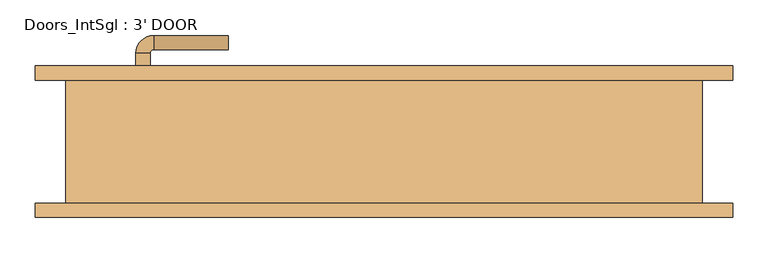
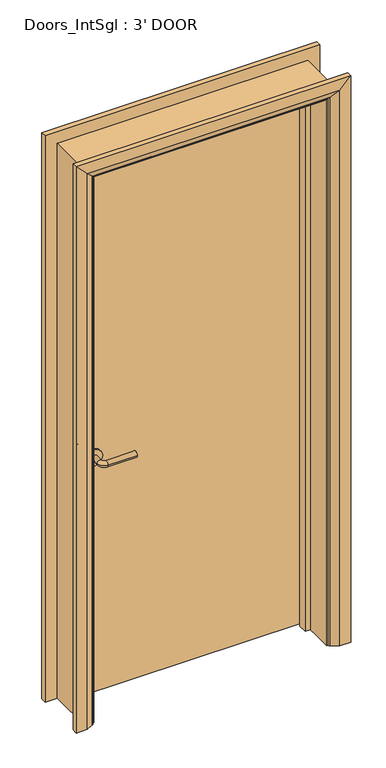
"""IFC4 building model written with IfcOpenShell, lengths in millimetres: door geometry, Doors_IntSgl : 3' DOOR."""

from ifc_helpers import new_model, si_unit, point, frame, frame_2d, origin, place, context, project, spatial, polyline, circle_curve, ellipse_curve, trimmed, segment, composite_curve, outline, extrude, faceted_brep, source, transform, mapped, element, save
from ifc_brep_helpers import plane_surface, cylinder_surface, revolved_surface, advanced_brep


def doors_intsgl_3_door_f61d7fb9(model_context):
    return source(origin(), model_context, "Body", "SolidModel", [
        advanced_brep(
        [(-350.2, 40.868, 900.0), (-330.2, 40.868, 900.0), (-330.2, 10.868, 900.0), (-350.2, 10.868, 900.0), (-325.2, 5.868, 900.0), (-325.2, -14.132, 900.0), (-220.2, -14.132, 900.0), (-220.2, 5.868, 900.0)],
        [
            (0, 1, circle_curve(frame((-340.2, 40.868, 900.0), z_axis=(0.0, 1.0, 0.0), x_axis=(1.0, 0.0, 0.0)), 10.0)),
            (1, 0, circle_curve(frame((-340.2, 40.868, 900.0), z_axis=(0.0, 1.0, 0.0), x_axis=(1.0, 0.0, 0.0)), 10.0)),
            (1, 2),
            (2, 3, circle_curve(frame((-340.2, 10.868, 900.0), z_axis=(0.0, 1.0, 0.0), x_axis=(1.0, 0.0, 0.0)), 10.0)),
            (3, 0),
            (3, 2, circle_curve(frame((-340.2, 10.868, 900.0), z_axis=(0.0, 1.0, 0.0), x_axis=(1.0, 0.0, 0.0)), 10.0)),
            (4, 5, circle_curve(frame((-325.2, -4.132, 900.0), z_axis=(-1.0, 0.0, 0.0), x_axis=(0.0, 1.0, 0.0)), 10.0)),
            (5, 3, circle_curve(frame((-325.2, 10.868, 900.0), z_axis=(0.0, 0.0, -1.0), x_axis=(-1.0, 0.0, 0.0)), 25.0)),
            (2, 4, circle_curve(frame((-325.2, 10.868, 900.0), z_axis=(0.0, 0.0, 1.0), x_axis=(-1.0, 0.0, 0.0)), 5.0)),
            (5, 4, circle_curve(frame((-325.2, -4.132, 900.0), z_axis=(-1.0, 0.0, 0.0), x_axis=(0.0, 1.0, 0.0)), 10.0)),
            (6, 7, circle_curve(frame((-220.2, -4.132, 900.0), z_axis=(1.0, 0.0, 0.0), x_axis=(0.0, 1.0, 0.0)), 10.0)),
            (7, 6, circle_curve(frame((-220.2, -4.132, 900.0), z_axis=(1.0, 0.0, 0.0), x_axis=(0.0, 1.0, 0.0)), 10.0)),
            (4, 7),
            (6, 5),
        ],
        [
            plane_surface(frame((-340.2, 40.868, 900.0), z_axis=(0.0, 1.0, 0.0), x_axis=(0.0, 0.0, 1.0))),
            cylinder_surface(frame((-340.2, 40.868, 900.0), z_axis=(0.0, 1.0, 0.0), x_axis=(1.0, 0.0, 0.0)), 10.0),
            revolved_surface(trimmed(ellipse_curve(frame((-340.2, 10.868, 900.0), z_axis=(0.0, -1.0, 0.0), x_axis=(1.0, 0.0, 0.0)), 10.0, 10.0), [point((-350.2, 10.868, 900.0))], [point((-330.2, 10.868, 900.0))], True, "CARTESIAN"), (-325.2, 10.868, 900.0), (0.0, 0.0, -1.0)),
            revolved_surface(trimmed(ellipse_curve(frame((-340.2, 10.868, 900.0), z_axis=(0.0, -1.0, 0.0), x_axis=(1.0, 0.0, 0.0)), 10.0, 10.0), [point((-330.2, 10.868, 900.0))], [point((-350.2, 10.868, 900.0))], True, "CARTESIAN"), (-325.2, 10.868, 900.0), (0.0, 0.0, -1.0)),
            plane_surface(frame((-220.2, -4.132, 900.0), z_axis=(1.0, 0.0, 0.0), x_axis=(0.0, 0.0, 1.0))),
            cylinder_surface(frame((-325.2, -4.132, 900.0), z_axis=(-1.0, 0.0, 0.0), x_axis=(0.0, 1.0, 0.0)), 10.0),
        ],
        [
            (0, [[1, 2]]),
            (1, [[3, 4, 5, -2]]),
            (1, [[-5, 6, -3, -1]]),
            (2, [[7, 8, -4, 9]]),
            (3, [[10, -9, -6, -8]]),
            (4, [[11, 12]]),
            (5, [[13, -11, 14, -7]]),
            (5, [[-14, -12, -13, -10]]),
        ],
    ),
        extrude(outline(composite_curve([segment(trimmed(circle_curve(frame_2d((900.0, -342.7)), 30.0), [point((900.0, -372.7))], [point((900.0, -312.7))], False, "CARTESIAN"), True, "CONTINUOUS"), segment(trimmed(circle_curve(frame_2d((900.0, -342.7)), 30.0), [point((900.0, -312.7))], [point((900.0, -372.7))], False, "CARTESIAN"), True, "CONTINUOUS")], self_intersect=False)), frame((0.0, 40.868, 0.0), z_axis=(0.0, 1.0, 0.0), x_axis=(0.0, 0.0, 1.0)), (0.0, 0.0, 1.0), 8.0),
        advanced_brep(
        [(-350.2, 94.868, 900.0), (-330.2, 94.868, 900.0), (-350.2, 124.868, 900.0), (-330.2, 124.868, 900.0), (-325.2, 129.868, 900.0), (-325.2, 149.868, 900.0), (-220.2, 149.868, 900.0), (-220.2, 129.868, 900.0)],
        [
            (0, 1, circle_curve(frame((-340.2, 94.868, 900.0), z_axis=(0.0, -1.0, 0.0), x_axis=(1.0, 0.0, 0.0)), 10.0)),
            (1, 0, circle_curve(frame((-340.2, 94.868, 900.0), z_axis=(0.0, -1.0, 0.0), x_axis=(1.0, 0.0, 0.0)), 10.0)),
            (0, 2),
            (2, 3, circle_curve(frame((-340.2, 124.868, 900.0), z_axis=(0.0, -1.0, 0.0), x_axis=(1.0, 0.0, 0.0)), 10.0)),
            (3, 1),
            (3, 2, circle_curve(frame((-340.2, 124.868, 900.0), z_axis=(0.0, -1.0, 0.0), x_axis=(1.0, 0.0, 0.0)), 10.0)),
            (4, 3, circle_curve(frame((-325.2, 124.868, 900.0), z_axis=(0.0, 0.0, 1.0), x_axis=(-1.0, 0.0, 0.0)), 5.0)),
            (2, 5, circle_curve(frame((-325.2, 124.868, 900.0), z_axis=(0.0, 0.0, -1.0), x_axis=(-1.0, 0.0, 0.0)), 25.0)),
            (5, 4, circle_curve(frame((-325.2, 139.868, 900.0), z_axis=(-1.0, 0.0, 0.0), x_axis=(0.0, -1.0, 0.0)), 10.0)),
            (4, 5, circle_curve(frame((-325.2, 139.868, 900.0), z_axis=(-1.0, 0.0, 0.0), x_axis=(0.0, -1.0, 0.0)), 10.0)),
            (6, 7, circle_curve(frame((-220.2, 139.868, 900.0), z_axis=(1.0, 0.0, 0.0), x_axis=(0.0, -1.0, 0.0)), 10.0)),
            (7, 6, circle_curve(frame((-220.2, 139.868, 900.0), z_axis=(1.0, 0.0, 0.0), x_axis=(0.0, -1.0, 0.0)), 10.0)),
            (5, 6),
            (7, 4),
        ],
        [
            plane_surface(frame((-340.2, 94.868, 900.0), z_axis=(0.0, -1.0, 0.0), x_axis=(0.0, 0.0, 1.0))),
            cylinder_surface(frame((-340.2, 94.868, 900.0), z_axis=(0.0, -1.0, 0.0), x_axis=(1.0, 0.0, 0.0)), 10.0),
            revolved_surface(trimmed(ellipse_curve(frame((-340.2, 124.868, 900.0), z_axis=(0.0, -1.0, 0.0), x_axis=(1.0, 0.0, 0.0)), 10.0, 10.0), [point((-350.2, 124.868, 900.0))], [point((-330.2, 124.868, 900.0))], True, "CARTESIAN"), (-325.2, 124.868, 900.0), (0.0, 0.0, -1.0)),
            revolved_surface(trimmed(ellipse_curve(frame((-340.2, 124.868, 900.0), z_axis=(0.0, -1.0, 0.0), x_axis=(1.0, 0.0, 0.0)), 10.0, 10.0), [point((-330.2, 124.868, 900.0))], [point((-350.2, 124.868, 900.0))], True, "CARTESIAN"), (-325.2, 124.868, 900.0), (0.0, 0.0, -1.0)),
            plane_surface(frame((-220.2, 139.868, 900.0), z_axis=(1.0, 0.0, 0.0), x_axis=(0.0, 0.0, 1.0))),
            cylinder_surface(frame((-325.2, 139.868, 900.0), z_axis=(-1.0, 0.0, 0.0), x_axis=(0.0, -1.0, 0.0)), 10.0),
        ],
        [
            (0, [[1, 2]]),
            (1, [[-1, 3, 4, 5]]),
            (1, [[-2, -5, 6, -3]]),
            (2, [[7, -4, 8, 9]]),
            (3, [[-8, -6, -7, 10]]),
            (4, [[11, 12]]),
            (5, [[-9, 13, -12, 14]]),
            (5, [[-10, -14, -11, -13]]),
        ],
    ),
        extrude(outline(composite_curve([segment(trimmed(circle_curve(frame_2d((900.0, -342.7)), 30.0), [point((900.0, -372.7))], [point((900.0, -312.7))], False, "CARTESIAN"), True, "CONTINUOUS"), segment(trimmed(circle_curve(frame_2d((900.0, -342.7)), 30.0), [point((900.0, -312.7))], [point((900.0, -372.7))], False, "CARTESIAN"), True, "CONTINUOUS")], self_intersect=False)), frame((0.0, 86.868, 0.0), z_axis=(0.0, 1.0, 0.0), x_axis=(0.0, 0.0, 1.0)), (0.0, 0.0, 1.0), 8.0),
        extrude(outline(polyline([(415.2, 48.868), (-415.2, 48.868), (-415.2, 86.868), (415.2, 86.868), (415.2, 48.868)])), frame((0.0, 0.0, 8.0), z_axis=(0.0, 0.0, 1.0), x_axis=(1.0, 0.0, 0.0)), (0.0, 0.0, 1.0), 2060.0),
        advanced_brep(
        [(492.2, 106.868, 0.0), (492.2, 86.868, 0.0), (422.2, 86.868, 0.0), (426.2, 92.868, 0.0), (452.2, 106.868, 0.0), (492.2, 106.868, 2145.0), (492.2, 86.868, 2145.0), (-492.2, 86.868, 2145.0), (-492.2, 86.868, 0.0), (-422.2, 86.868, 0.0), (-422.2, 86.868, 2075.0), (422.2, 86.868, 2075.0), (426.2, 92.868, 2079.0), (452.2, 106.868, 2105.0), (-452.2, 106.868, 2105.0), (-452.2, 106.868, 0.0), (-492.2, 106.868, 0.0), (-492.2, 106.868, 2145.0), (-426.2, 92.868, 0.0), (-426.2, 92.868, 2079.0)],
        [
            (0, 1),
            (1, 2),
            (2, 3, circle_curve(frame((430.2, 85.868, 0.0), z_axis=(0.0, 0.0, -1.0), x_axis=(1.0, 0.0, 0.0)), 8.0622577)),
            (3, 4),
            (4, 0),
            (0, 5),
            (5, 6),
            (6, 1),
            (6, 7),
            (7, 8),
            (8, 9),
            (9, 10),
            (10, 11),
            (11, 2),
            (11, 12, ellipse_curve(frame((430.2, 85.868, 2083.0), z_axis=(0.7071067811865475, 0.0, -0.7071067811865475), x_axis=(-0.7071067811865474, 0.0, -0.7071067811865476)), 11.4017543, 8.0622577)),
            (12, 3),
            (12, 13),
            (13, 4),
            (13, 14),
            (14, 15),
            (15, 16),
            (16, 17),
            (17, 5),
            (7, 17),
            (16, 8),
            (15, 18),
            (18, 9, circle_curve(frame((-430.2, 85.868, 0.0), z_axis=(0.0, 0.0, -1.0), x_axis=(-1.0, 0.0, 0.0)), 8.0622577)),
            (19, 10, ellipse_curve(frame((-430.2, 85.868, 2083.0), z_axis=(-0.7071067811865475, 0.0, -0.7071067811865475), x_axis=(-0.7071067811865474, 0.0, 0.7071067811865476)), 11.4017543, 8.0622577)),
            (18, 19),
            (14, 19),
            (19, 12),
        ],
        [
            plane_surface(frame((422.2, 86.868, 0.0), z_axis=(0.0, 0.0, -1.0), x_axis=(0.0, -1.0, 0.0))),
            plane_surface(frame((492.2, 106.868, 0.0), z_axis=(1.0, 0.0, 0.0), x_axis=(0.0, 0.0, 1.0))),
            plane_surface(frame((492.2, 86.868, 0.0), z_axis=(0.0, -1.0, 0.0), x_axis=(0.0, 0.0, 1.0))),
            cylinder_surface(frame((430.2, 85.868, 0.0), z_axis=(0.0, 0.0, -1.0), x_axis=(1.0, 0.0, 0.0)), 8.0622577),
            plane_surface(frame((426.2, 92.868, 0.0), z_axis=(-0.4740998230350126, 0.880471099922178, 0.0), x_axis=(0.0, 0.0, 1.0))),
            plane_surface(frame((452.2, 106.868, 0.0), z_axis=(0.0, 1.0, 0.0), x_axis=(0.0, 0.0, 1.0))),
            plane_surface(frame((-492.2, 106.868, 2145.0), z_axis=(-1.0, 0.0, 0.0), x_axis=(0.0, 0.0, -1.0))),
            plane_surface(frame((-422.2, 86.868, 0.0), z_axis=(0.0, 0.0, -1.0), x_axis=(0.0, -1.0, 0.0))),
            cylinder_surface(frame((-430.2, 85.868, 2075.0), z_axis=(0.0, 0.0, 1.0), x_axis=(-1.0, 0.0, 0.0)), 8.0622577),
            plane_surface(frame((-426.2, 92.868, 2079.0), z_axis=(0.47409982303501824, 0.8804710999221749, 0.0), x_axis=(0.0, 0.0, -1.0))),
            plane_surface(frame((492.2, 106.868, 2145.0), z_axis=(0.0, 0.0, 1.0), x_axis=(-1.0, 0.0, 0.0))),
            cylinder_surface(frame((422.2, 85.868, 2083.0), z_axis=(1.0, 0.0, 0.0), x_axis=(0.0, 0.0, 1.0)), 8.0622577),
            plane_surface(frame((426.2, 92.868, 2079.0), z_axis=(0.0, 0.8804710999221764, -0.4740998230350154), x_axis=(-1.0, 0.0, 0.0))),
        ],
        [
            (0, [[1, 2, 3, 4, 5]]),
            (1, [[-1, 6, 7, 8]]),
            (2, [[-2, -8, 9, 10, 11, 12, 13, 14]]),
            (3, [[-3, -14, 15, 16]]),
            (4, [[-4, -16, 17, 18]]),
            (5, [[-5, -18, 19, 20, 21, 22, 23, -6]]),
            (6, [[24, -22, 25, -10]]),
            (7, [[-21, 26, 27, -11, -25]]),
            (8, [[28, -12, -27, 29]]),
            (9, [[30, -29, -26, -20]]),
            (10, [[-7, -23, -24, -9]]),
            (11, [[-15, -13, -28, 31]]),
            (12, [[-17, -31, -30, -19]]),
        ],
    ),
        extrude(outline(polyline([(0.0, -417.2), (0.0, -398.2), (2051.0, -398.2), (2051.0, 398.2), (0.0, 398.2), (0.0, 417.2), (2070.0, 417.2), (2070.0, -417.2), (0.0, -417.2)])), frame((0.0, 14.868, 0.0), z_axis=(0.0, 1.0, 0.0), x_axis=(0.0, 0.0, 1.0)), (0.0, 0.0, 1.0), 32.0),
        advanced_brep(
        [(-492.2, -106.868, 0.0), (-492.2, -86.868, 0.0), (-422.2, -86.868, 0.0), (-426.2, -92.868, 0.0), (-452.2, -106.868, 0.0), (-492.2, -106.868, 2145.0), (-492.2, -86.868, 2145.0), (-422.2, -86.868, 2075.0), (-426.2, -92.868, 2079.0), (-452.2, -106.868, 2105.0), (492.2, -106.868, 0.0), (452.2, -106.868, 0.0), (426.2, -92.868, 0.0), (422.2, -86.868, 0.0), (492.2, -86.868, 0.0), (492.2, -106.868, 2145.0), (452.2, -106.868, 2105.0), (426.2, -92.868, 2079.0), (422.2, -86.868, 2075.0), (492.2, -86.868, 2145.0)],
        [
            (0, 1),
            (1, 2),
            (2, 3, circle_curve(frame((-430.2, -85.868, 0.0), z_axis=(0.0, 0.0, -1.0), x_axis=(-1.0, 0.0, 0.0)), 8.0622577)),
            (3, 4),
            (4, 0),
            (0, 5),
            (5, 6),
            (6, 1),
            (6, 7),
            (7, 2),
            (7, 8, ellipse_curve(frame((-430.2, -85.868, 2083.0), z_axis=(-0.7071067811865475, 0.0, -0.7071067811865475), x_axis=(0.7071067811865474, 0.0, -0.7071067811865476)), 11.4017543, 8.0622577)),
            (8, 3),
            (8, 9),
            (9, 4),
            (9, 5),
            (10, 11),
            (11, 12),
            (12, 13, circle_curve(frame((430.2, -85.868, 0.0), z_axis=(0.0, 0.0, -1.0), x_axis=(1.0, 0.0, 0.0)), 8.0622577)),
            (13, 14),
            (14, 10),
            (15, 16),
            (16, 11),
            (10, 15),
            (16, 17),
            (17, 12),
            (17, 18, ellipse_curve(frame((430.2, -85.868, 2083.0), z_axis=(0.7071067811865475, 0.0, -0.7071067811865475), x_axis=(0.7071067811865474, 0.0, 0.7071067811865476)), 11.4017543, 8.0622577)),
            (18, 13),
            (18, 19),
            (19, 14),
            (19, 15),
            (5, 15),
            (19, 6),
            (18, 7),
            (17, 8),
            (16, 9),
        ],
        [
            plane_surface(frame((-422.2, -159.6690989, 0.0), z_axis=(0.0, 0.0, -1.0), x_axis=(1.0, 0.0, 0.0))),
            plane_surface(frame((-492.2, -106.868, 0.0), z_axis=(-1.0, 0.0, 0.0), x_axis=(0.0, 0.0, 1.0))),
            plane_surface(frame((-492.2, -86.868, 0.0), z_axis=(0.0, 1.0, 0.0), x_axis=(0.0, 0.0, 1.0))),
            cylinder_surface(frame((-430.2, -85.868, 0.0), z_axis=(0.0, 0.0, -1.0), x_axis=(-1.0, 0.0, 0.0)), 8.0622577),
            plane_surface(frame((-426.2, -92.868, 0.0), z_axis=(0.4740998230350183, -0.8804710999221749, 0.0), x_axis=(0.0, 0.0, 1.0))),
            plane_surface(frame((-452.2, -106.868, 0.0), z_axis=(0.0, -1.0, 0.0), x_axis=(0.0, 0.0, 1.0))),
            plane_surface(frame((422.2, -159.6690989, 0.0), z_axis=(0.0, 0.0, -1.0), x_axis=(-1.0, 0.0, 0.0))),
            plane_surface(frame((452.2, -106.868, 2105.0), z_axis=(0.0, -1.0, 0.0), x_axis=(0.0, 0.0, -1.0))),
            plane_surface(frame((426.2, -92.868, 2079.0), z_axis=(-0.4740998230350183, -0.8804710999221749, 0.0), x_axis=(0.0, 0.0, -1.0))),
            cylinder_surface(frame((430.2, -85.868, 2075.0), z_axis=(0.0, 0.0, 1.0), x_axis=(1.0, 0.0, 0.0)), 8.0622577),
            plane_surface(frame((492.2, -86.868, 2145.0), z_axis=(0.0, 1.0, 0.0), x_axis=(0.0, 0.0, -1.0))),
            plane_surface(frame((492.2, -106.868, 2145.0), z_axis=(1.0, 0.0, 0.0), x_axis=(0.0, 0.0, -1.0))),
            plane_surface(frame((-492.2, -106.868, 2145.0), z_axis=(0.0, 0.0, 1.0), x_axis=(1.0, 0.0, 0.0))),
            plane_surface(frame((-492.2, -86.868, 2145.0), z_axis=(0.0, 1.0, 0.0), x_axis=(1.0, 0.0, 0.0))),
            cylinder_surface(frame((-422.2, -85.868, 2083.0), z_axis=(-1.0, 0.0, 0.0), x_axis=(0.0, 0.0, 1.0)), 8.0622577),
            plane_surface(frame((-426.2, -92.868, 2079.0), z_axis=(0.0, -0.8804710999221749, -0.4740998230350183), x_axis=(1.0, 0.0, 0.0))),
            plane_surface(frame((-452.2, -106.868, 2105.0), z_axis=(0.0, -1.0, 0.0), x_axis=(1.0, 0.0, 0.0))),
        ],
        [
            (0, [[1, 2, 3, 4, 5]]),
            (1, [[-1, 6, 7, 8]]),
            (2, [[-2, -8, 9, 10]]),
            (3, [[-3, -10, 11, 12]]),
            (4, [[-4, -12, 13, 14]]),
            (5, [[-5, -14, 15, -6]]),
            (6, [[16, 17, 18, 19, 20]]),
            (7, [[21, 22, -16, 23]]),
            (8, [[24, 25, -17, -22]]),
            (9, [[26, 27, -18, -25]]),
            (10, [[28, 29, -19, -27]]),
            (11, [[30, -23, -20, -29]]),
            (12, [[-7, 31, -30, 32]]),
            (13, [[-9, -32, -28, 33]]),
            (14, [[-11, -33, -26, 34]]),
            (15, [[-13, -34, -24, 35]]),
            (16, [[-15, -35, -21, -31]]),
        ],
    ),
        faceted_brep([(-417.2, 86.868, 0.0), (-417.2, -86.868, 0.0), (-449.2, -86.868, 0.0), (-449.2, 86.868, 0.0), (-417.2, 86.868, 2070.0), (-417.2, -86.868, 2070.0), (-449.2, -86.868, 2102.0), (-449.2, 86.868, 2102.0), (417.2, 86.868, 0.0), (449.2, 86.868, 0.0), (449.2, -86.868, 0.0), (417.2, -86.868, 0.0), (417.2, 86.868, 2070.0), (449.2, 86.868, 2102.0), (449.2, -86.868, 2102.0), (417.2, -86.868, 2070.0)], [[[0, 1, 2, 3]], [[1, 0, 4, 5]], [[2, 1, 5, 6]], [[3, 2, 6, 7]], [[0, 3, 7, 4]], [[8, 9, 10, 11]], [[12, 13, 9, 8]], [[13, 14, 10, 9]], [[14, 15, 11, 10]], [[15, 12, 8, 11]], [[5, 4, 12, 15]], [[6, 5, 15, 14]], [[7, 6, 14, 13]], [[4, 7, 13, 12]]]),
    ])


if __name__ == "__main__":
    model = new_model("IFC4")
    model_context = context("Model", 3, world=origin())
    ifc_project = project(units=[si_unit("LENGTHUNIT", "METRE", prefix="MILLI")], contexts=[model_context])
    site = spatial("IfcSite", under=ifc_project)
    building = spatial("IfcBuilding", under=site)
    placement = place(None, origin())
    doors_intsgl_3_door_shape = doors_intsgl_3_door_f61d7fb9(model_context)
    element("IfcDoor", 1, ObjectType="Doors_IntSgl : 3' DOOR", at=placement, inside=building, context=model_context, shape_type="MappedRepresentation", body=[
        mapped(doors_intsgl_3_door_shape, transform((0.0, 0.0, 0.0), x_axis=(1.0, 0.0, 0.0), y_axis=(0.0, 1.0, 0.0), z_axis=(0.0, 0.0, 1.0))),
    ])
    save(model, "model.ifc")

# Revit data of these elements
# Type "Doors_IntSgl : 3' DOOR"
#   Type Mark = "46"
#   Type Comments = "Internal Single"
#   Operation = "SingleSwingRight"
#   Manufacturer = "Revit"
#   Keynote = "L20"
#   Description = "Internal Single Door"
#   Analytic Construction = "Metal"
#   UnderCut = 0.026247 ft
#   Tolerance = 0.006562 ft
#   Thickness = 0.124672 ft
#   Thermal Resistance (R) = 0.270117 (m²·K)/W
#   Structural Tolerance = 0.026247 ft
#   StopDepth = 0.104987 ft
#   Stop Thickness = 0.062336 ft
#   Rough Width = 3.0 ft
#   Rough Height = 6.922572 ft
#   Height to Top Lock Rail = 3.28084 ft
#   Heat Transfer Coefficient (U) = 3.7021 W/(m²·K)
#   Handle Z Distance = 2.952756 ft
#   Handle X Distance = 0.246063 ft
#   Frame Thickness = 0.104987 ft
#   Door Panel Width = 2.724409 ft
#   Door Panel Thickness = 0.124672 ft
#   Door Panel Offset = 0.0 ft
#   Height = 6.922572 ft
#   Width = 3.0 ft
#   Door Panel Height = 6.75853 ft
#   Architrave Setback = 0.016404 ft
#   Vis - Ironmongery = yes
#   Material Ironmongery = Door - Handle
#   Material Frame = Door - Frame/Mullion (1)
#   Material Door = Door - Panel
#   Material Architrave = Door - Architrave
#   Visual Light Transmittance = 0
#   Solar Heat Gain Coefficient = 0
#   Function = (empty or 0)
#   Wall Closure = (empty or 0)
# Element 1 (IfcDoor, "Doors_IntSgl : 3' DOOR")
#   Materials on its faces: "Door - Architrave", "Door - Handle", "Door - Frame/Mullion (1)", "Door - Panel"
# Materials
#   "Door - Handle": colour RGB 0 0 0, transparency 0, Keynote = "P21", Cost = 0
#   "Door - Frame/Mullion (1)": class "Wood", colour RGB 212 179 113, transparency 0, Keynote = "L20", Cost = 0
#   "Door - Panel": class "Wood", colour RGB 210 159 95, transparency 0, Keynote = "L20", Cost = 0
#   "Door - Architrave": class "Wood", colour RGB 154 90 5, transparency 0, Keynote = "P20", Cost = 0
